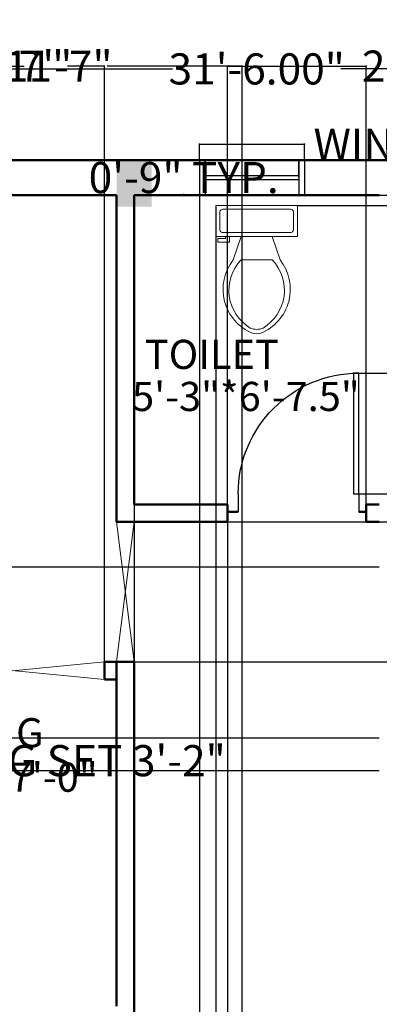
# Model space of a CAD drawing. Units: inches. Extents: x 9717 to 10218, y 17835 to 18358.
# Tile 3 of 4: x 9901 to 9993, y 18104 to 18358. Entities that reach past the tile are written whole.
import ezdxf

# ---------------------------------------------------------------- set-up
doc = ezdxf.new("R2010")
doc.units = ezdxf.units.IN
for name, color, linetype, lineweight in [('A-AREA-IDEN', 3, 'Continuous', 25), ('A-FLOR-FIXT', 2, 'Continuous', 18), ('ARCHES', 5, 'Continuous', 18), ('COLUMN', 7, 'Continuous', 35), ('DIMENSIONS', 3, 'Continuous', 18), ('DOORS', 1, 'Continuous', 25), ('WALLS', 7, 'Continuous', 50), ('WINDOWS', 4, 'Continuous', 25)]:
    doc.layers.add(name, color=color, linetype=linetype, lineweight=lineweight)
doc.styles.get("Standard").update_dxf_attribs({"font": 'arial.ttf'})
doc.dimstyles.get("Standard").update_dxf_attribs({"dimtxt": 8, "dimasz": 0.18, "dimexe": 0.18, "dimexo": 0.0625, "dimgap": 0.09, "dimtad": 0, "dimtih": 1, "dimtoh": 1, "dimzin": 0, "dimdsep": 46, "dimlunit": 3, "dimtxsty": 'Standard', "dimcen": 0.09, "dimadec": 0, "dimazin": 0, "dimtfac": 1, "dimtofl": 0, "dimtmove": 0, "dimatfit": 3, "dimfxl": 1, "dimtolj": 1, "dimtzin": 0, "dimarcsym": 0})

# ---------------------------------------------------------------- blocks, each defined once
blk = doc.blocks.new('*U2')
for p, q in [((0, 0), (0, -6)), ((40, 0), (40, -6))]:
    blk.add_line(p, q)
blk.add_lwpolyline([(0, 0), (0, 40), (1.75, 40), (1.75, 0)], close=True)
blk.add_arc((0, 0), 40, 0, 90)
blk = doc.blocks.new('Toilet - top')
for p, q in [((9.5, -6), (9.5, -2)), ((-10, -8.5), (-8, -8.5)), ((-10, -9.5), (-10, -8.5)), ((-7, -9.5), (-10, -9.5)), ((-8, -8.5), (-8, -8)), ((-7, -8), (-7, -9.5)), ((-4, -8), (-6, -14)), ((4, -8), (6, -14)), ((4, -14), (-4, -14))]:
    blk.add_line(p, q)
blk.add_lwpolyline([(10.5, -8), (10.5, 0), (-10.5, 0), (-10.5, -8)], close=True)
for points in [[(-9.5, -2), (-9.5, -6)], [(8.5, -1), (-8.5, -1)], [(-8.5, -7), (8.5, -7)]]:
    blk.add_lwpolyline(points)
for centre, radius, start, end in [((-8.62, -1.88), 0.884, 81.8699, 188.1301), ((8.62, -1.88), 0.884, 351.8699, 98.1301), ((-8.62, -6.12), 0.884, 171.8699, 278.1301), ((8.62, -6.12), 0.884, 261.8699, 8.1301), ((3.52, -21.58), 12.17, 141.4691, 247.9714), ((4.2, -21.82), 11.33, 136.3677, 238.9468), ((-3.52, -21.58), 12.17, 292.0284, 38.5307), ((-4.2, -21.82), 11.33, 301.053, 43.6321), ((0, -27.88), 4, 245.7318, 294.2682), ((0, -29), 4, 254.8605, 285.1395)]:
    blk.add_arc(centre, radius, start, end)
blk = doc.blocks.new('*D8')
at = {"layer": 'Defpoints', "color": 0, "transparency": 16777216}
for p in [(10150.76, 18344.92), (9772.76, 18321.49), (10150.76, 18321.49)]:
    blk.add_point(p, dxfattribs=at)
at = {"layer": 'DIMENSIONS', "color": 0, "lineweight": -2, "transparency": 16777216}
for p, q in [((9772.76, 18321.55), (9772.76, 18345.1)), ((9772.94, 18344.92), (9940.16, 18344.92)), ((10150.58, 18344.92), (9983.36, 18344.92)), ((10150.76, 18321.55), (10150.76, 18345.1))]:
    blk.add_line(p, q, dxfattribs=at)
at = {"layer": 'DIMENSIONS', "color": 0, "transparency": 16777216}
for points in [[(9772.94, 18344.95), (9772.94, 18344.89), (9772.76, 18344.92)], [(10150.58, 18344.95), (10150.58, 18344.89), (10150.76, 18344.92)]]:
    blk.add_solid(points, dxfattribs=at)
at = {"layer": 'DIMENSIONS', "color": 0, "transparency": 16777216, "insert": (9961.76, 18344.92), "char_height": 8, "attachment_point": 5}
blk.add_mtext('\\A1;31\'-6.00"', dxfattribs=at)
blk = doc.blocks.new('WIN-24IN')
for p, q in [((1.5, 9), (0, 9)), ((0, 9), (0, 0)), ((1.5, 4.5), (1.5, 9)), ((1.5, 9), (1.5, 0)), ((25.5, 4.5), (25.5, 9)), ((25.5, 9), (25.5, 0)), ((25.5, 9), (27, 9)), ((27, 9), (27, 0)), ((1.5, 5), (25.5, 5)), ((1.5, 4), (25.5, 4)), ((0, 0), (1.5, 0)), ((27, 0), (25.5, 0))]:
    blk.add_line(p, q)
blk = doc.blocks.new('COL-12X9IN')
h = blk.add_hatch(color=256)
h.dxf.hatch_style = 1
h.paths.add_polyline_path([(12, 0), (12, 9), (0, 9), (0, 0)])
blk = doc.blocks.new('*D18')
at = {"layer": 'Defpoints', "color": 0, "transparency": 16777216}
for p in [(9974.05, 18325.54), (9947.05, 18321.49), (9974.05, 18321.49)]:
    blk.add_point(p, dxfattribs=at)
at = {"layer": 'DIMENSIONS', "color": 0, "lineweight": -2, "transparency": 16777216}
for p, q in [((9947.05, 18321.55), (9947.05, 18325.72)), ((9947.23, 18325.54), (9973.87, 18325.54)), ((9974.05, 18321.55), (9974.05, 18325.72)), ((9974.05, 18325.54), (9974.23, 18325.54))]:
    blk.add_line(p, q, dxfattribs=at)
at = {"layer": 'DIMENSIONS', "color": 0, "transparency": 16777216}
for points in [[(9947.23, 18325.57), (9947.23, 18325.51), (9947.05, 18325.54)], [(9973.87, 18325.57), (9973.87, 18325.51), (9974.05, 18325.54)]]:
    blk.add_solid(points, dxfattribs=at)
at = {"layer": 'DIMENSIONS', "color": 0, "transparency": 16777216, "insert": (10024.94, 18325.54), "char_height": 8, "attachment_point": 5}
blk.add_mtext('\\A1;WINDOW 2\'-3" TYP.', dxfattribs=at)
blk = doc.blocks.new('*D19')
at = {"layer": 'Defpoints', "color": 0, "transparency": 16777216}
for p in [(9943, 18321.49), (9947.05, 18321.49), (9947.05, 18312.49)]:
    blk.add_point(p, dxfattribs=at)
at = {"layer": 'DIMENSIONS', "color": 0, "lineweight": -2, "transparency": 16777216}
for p, q in [((9946.99, 18321.49), (9942.82, 18321.49)), ((9943, 18321.31), (9943, 18321.17)), ((9946.99, 18312.49), (9942.82, 18312.49)), ((9943, 18312.67), (9943, 18312.82))]:
    blk.add_line(p, q, dxfattribs=at)
at = {"layer": 'DIMENSIONS', "color": 0, "transparency": 16777216}
for points in [[(9942.97, 18321.31), (9943.03, 18321.31), (9943, 18321.49)], [(9942.97, 18312.67), (9943.03, 18312.67), (9943, 18312.49)]]:
    blk.add_solid(points, dxfattribs=at)
at = {"layer": 'DIMENSIONS', "color": 0, "transparency": 16777216, "insert": (9943, 18316.99), "char_height": 8, "attachment_point": 5}
blk.add_mtext('\\A1;0\'-9" TYP.', dxfattribs=at)
blk = doc.blocks.new('*D28')
at = {"layer": 'Defpoints', "color": 0, "transparency": 16777216}
for p in [(9866.73, 18167.12), (9828.75, 18161.43), (9866.73, 18161.43)]:
    blk.add_point(p, dxfattribs=at)
at = {"layer": 'DIMENSIONS', "color": 0, "lineweight": -2, "transparency": 16777216}
for p, q in [((9828.75, 18161.49), (9828.75, 18167.3)), ((9828.93, 18167.12), (9866.55, 18167.12)), ((9866.73, 18161.49), (9866.73, 18167.3)), ((9866.73, 18167.12), (9866.91, 18167.12))]:
    blk.add_line(p, q, dxfattribs=at)
at = {"layer": 'DIMENSIONS', "color": 0, "transparency": 16777216}
for points in [[(9828.93, 18167.15), (9828.93, 18167.09), (9828.75, 18167.12)], [(9866.55, 18167.15), (9866.55, 18167.09), (9866.73, 18167.12)]]:
    blk.add_solid(points, dxfattribs=at)
at = {"layer": 'DIMENSIONS', "color": 0, "transparency": 16777216, "insert": (9910.97, 18167.12), "char_height": 8, "attachment_point": 5}
blk.add_mtext('\\A1;DINING SET 3\'-2"', dxfattribs=at)
blk = doc.blocks.new('*D33')
at = {"layer": 'Defpoints', "color": 0, "transparency": 16777216}
for p in [(9958.06, 18345.64), (9867.28, 17970.49), (9958.06, 17970.49)]:
    blk.add_point(p, dxfattribs=at)
at = {"layer": 'DIMENSIONS', "color": 0, "lineweight": -2, "transparency": 16777216}
for p, q in [((9867.28, 17970.55), (9867.28, 18345.82)), ((9958.06, 17970.55), (9958.06, 18345.82)), ((9867.46, 18345.64), (9901.98, 18345.64)), ((9957.88, 18345.64), (9923.36, 18345.64))]:
    blk.add_line(p, q, dxfattribs=at)
at = {"layer": 'DIMENSIONS', "color": 0, "transparency": 16777216}
for points in [[(9867.46, 18345.67), (9867.46, 18345.61), (9867.28, 18345.64)], [(9957.88, 18345.67), (9957.88, 18345.61), (9958.06, 18345.64)]]:
    blk.add_solid(points, dxfattribs=at)
at = {"layer": 'DIMENSIONS', "color": 0, "transparency": 16777216, "insert": (9912.67, 18345.64), "char_height": 8, "attachment_point": 5}
blk.add_mtext('\\A1;7\'-7"', dxfattribs=at)
blk = doc.blocks.new('*D41')
at = {"layer": 'Defpoints', "color": 0, "transparency": 16777216}
for p in [(9930.26, 18312.49), (9947.05, 18312.49), (9947.05, 17847.34)]:
    blk.add_point(p, dxfattribs=at)
at = {"layer": 'DIMENSIONS', "color": 0, "lineweight": -2, "transparency": 16777216}
for p, q in [((9930.26, 18312.43), (9930.26, 17847.16)), ((9947.05, 18312.43), (9947.05, 17847.16)), ((9930.44, 17847.34), (9946.87, 17847.34)), ((9947.05, 17847.34), (9947.23, 17847.34))]:
    blk.add_line(p, q, dxfattribs=at)
at = {"layer": 'DIMENSIONS', "color": 0, "transparency": 16777216}
for points in [[(9930.44, 17847.37), (9930.44, 17847.31), (9930.26, 17847.34)], [(9946.87, 17847.37), (9946.87, 17847.31), (9947.05, 17847.34)]]:
    blk.add_solid(points, dxfattribs=at)
at = {"layer": 'DIMENSIONS', "color": 0, "transparency": 16777216, "insert": (9957.58, 17847.34), "char_height": 8, "attachment_point": 5}
blk.add_mtext('\\A1;1\'-5"', dxfattribs=at)
blk = doc.blocks.new('*D49')
at = {"layer": 'Defpoints', "color": 0, "transparency": 16777216}
for p in [(9922.68, 18345.64), (9875.9, 18192.49), (9922.68, 18192.49)]:
    blk.add_point(p, dxfattribs=at)
at = {"layer": 'DIMENSIONS', "color": 0, "lineweight": -2, "transparency": 16777216}
for p, q in [((9875.9, 18192.55), (9875.9, 18345.82)), ((9922.68, 18192.55), (9922.68, 18345.82)), ((9876.08, 18345.64), (9885.46, 18345.64)), ((9922.5, 18345.64), (9913.12, 18345.64))]:
    blk.add_line(p, q, dxfattribs=at)
at = {"layer": 'DIMENSIONS', "color": 0, "transparency": 16777216}
for points in [[(9876.08, 18345.67), (9876.08, 18345.61), (9875.9, 18345.64)], [(9922.5, 18345.67), (9922.5, 18345.61), (9922.68, 18345.64)]]:
    blk.add_solid(points, dxfattribs=at)
at = {"layer": 'DIMENSIONS', "color": 0, "transparency": 16777216, "insert": (9899.29, 18345.64), "char_height": 8, "attachment_point": 5}
blk.add_mtext('\\A1;3\'-11"', dxfattribs=at)
blk = doc.blocks.new('*D50')
at = {"layer": 'Defpoints', "color": 0, "transparency": 16777216}
for p in [(9930.26, 18228.49), (10174.91, 18228.49), (9930.26, 18192.49)]:
    blk.add_point(p, dxfattribs=at)
at = {"layer": 'DIMENSIONS', "color": 0, "lineweight": -2, "transparency": 16777216}
for p, q in [((9930.32, 18228.49), (10175.09, 18228.49)), ((10174.91, 18228.31), (10174.91, 18214.67)), ((10174.91, 18192.67), (10174.91, 18206.31)), ((9930.32, 18192.49), (10175.09, 18192.49))]:
    blk.add_line(p, q, dxfattribs=at)
at = {"layer": 'DIMENSIONS', "color": 0, "transparency": 16777216}
for points in [[(10174.88, 18228.31), (10174.94, 18228.31), (10174.91, 18228.49)], [(10174.88, 18192.67), (10174.94, 18192.67), (10174.91, 18192.49)]]:
    blk.add_solid(points, dxfattribs=at)
at = {"layer": 'DIMENSIONS', "color": 0, "transparency": 16777216, "insert": (10174.91, 18210.49), "char_height": 8, "attachment_point": 5}
blk.add_mtext('\\A1;3\'-0"', dxfattribs=at)
blk = doc.blocks.new('*D51')
at = {"layer": 'Defpoints', "color": 0, "transparency": 16777216}
for p in [(9989.89, 18345.64), (9954.27, 18232.99), (9989.89, 18232.99)]:
    blk.add_point(p, dxfattribs=at)
at = {"layer": 'DIMENSIONS', "color": 0, "lineweight": -2, "transparency": 16777216}
for p, q in [((9954.27, 18233.05), (9954.27, 18345.82)), ((9989.89, 18233.05), (9989.89, 18345.82)), ((9954.45, 18345.64), (9989.71, 18345.64)), ((9989.89, 18345.64), (9990.07, 18345.64))]:
    blk.add_line(p, q, dxfattribs=at)
at = {"layer": 'DIMENSIONS', "color": 0, "transparency": 16777216}
for points in [[(9954.45, 18345.67), (9954.45, 18345.61), (9954.27, 18345.64)], [(9989.71, 18345.67), (9989.71, 18345.61), (9989.89, 18345.64)]]:
    blk.add_solid(points, dxfattribs=at)
at = {"layer": 'DIMENSIONS', "color": 0, "transparency": 16777216, "insert": (10013.29, 18345.64), "char_height": 8, "attachment_point": 5}
blk.add_mtext('\\A1;2\'-11 1/2"', dxfattribs=at)
blk = doc.blocks.new('*D52')
at = {"layer": 'Defpoints', "color": 0, "transparency": 16777216}
for p in [(9748.61, 18216.87), (9993.26, 18216.87), (9993.26, 18172.92)]:
    blk.add_point(p, dxfattribs=at)
at = {"layer": 'DIMENSIONS', "color": 0, "lineweight": -2, "transparency": 16777216}
for p, q in [((9993.2, 18216.87), (9748.43, 18216.87)), ((9748.61, 18216.69), (9748.61, 18199.08)), ((9748.61, 18173.1), (9748.61, 18190.72)), ((9993.2, 18172.92), (9748.43, 18172.92))]:
    blk.add_line(p, q, dxfattribs=at)
at = {"layer": 'DIMENSIONS', "color": 0, "transparency": 16777216}
for points in [[(9748.58, 18216.69), (9748.64, 18216.69), (9748.61, 18216.87)], [(9748.58, 18173.1), (9748.64, 18173.1), (9748.61, 18172.92)]]:
    blk.add_solid(points, dxfattribs=at)
at = {"layer": 'DIMENSIONS', "color": 0, "transparency": 16777216, "insert": (9748.61, 18194.9), "char_height": 8, "attachment_point": 5}
blk.add_mtext('\\A1;3\'-8"', dxfattribs=at)
blk = doc.blocks.new('*D56')
at = {"layer": 'Defpoints', "color": 0, "transparency": 16777216}
for p in [(9986.65, 18266.74), (10174.91, 18266.74), (9986.65, 18235.74)]:
    blk.add_point(p, dxfattribs=at)
at = {"layer": 'DIMENSIONS', "color": 0, "lineweight": -2, "transparency": 16777216}
for p, q in [((9986.71, 18266.74), (10175.09, 18266.74)), ((10174.91, 18266.56), (10174.91, 18255.34)), ((10174.91, 18235.92), (10174.91, 18247.13)), ((9986.71, 18235.74), (10175.09, 18235.74))]:
    blk.add_line(p, q, dxfattribs=at)
at = {"layer": 'DIMENSIONS', "color": 0, "transparency": 16777216}
for points in [[(10174.88, 18266.56), (10174.94, 18266.56), (10174.91, 18266.74)], [(10174.88, 18235.92), (10174.94, 18235.92), (10174.91, 18235.74)]]:
    blk.add_solid(points, dxfattribs=at)
at = {"layer": 'DIMENSIONS', "color": 0, "transparency": 16777216, "insert": (10174.91, 18251.24), "char_height": 8, "attachment_point": 5}
blk.add_mtext('\\A1;2\'-7"', dxfattribs=at)
blk = doc.blocks.new('*D58')
at = {"layer": 'Defpoints', "color": 0, "transparency": 16777216}
for p in [(9930.26, 18232.99), (9954.27, 18232.99), (9954.27, 17847.34)]:
    blk.add_point(p, dxfattribs=at)
at = {"layer": 'DIMENSIONS', "color": 0, "lineweight": -2, "transparency": 16777216}
for p, q in [((9930.26, 18232.93), (9930.26, 17847.16)), ((9954.27, 18232.93), (9954.27, 17847.16)), ((9930.44, 17847.34), (9931.48, 17847.34)), ((9954.09, 17847.34), (9953.06, 17847.34))]:
    blk.add_line(p, q, dxfattribs=at)
at = {"layer": 'DIMENSIONS', "color": 0, "transparency": 16777216}
for points in [[(9930.44, 17847.37), (9930.44, 17847.31), (9930.26, 17847.34)], [(9954.09, 17847.37), (9954.09, 17847.31), (9954.27, 17847.34)]]:
    blk.add_solid(points, dxfattribs=at)
at = {"layer": 'DIMENSIONS', "color": 0, "transparency": 16777216, "insert": (9942.27, 17847.34), "char_height": 8, "attachment_point": 5}
blk.add_mtext('\\A1;2\'-0"', dxfattribs=at)
blk = doc.blocks.new('*D61')
at = {"layer": 'Defpoints', "color": 0, "transparency": 16777216}
for p in [(9748.61, 18172.92), (9993.26, 18172.92), (9993.26, 18164.49)]:
    blk.add_point(p, dxfattribs=at)
at = {"layer": 'DIMENSIONS', "color": 0, "lineweight": -2, "transparency": 16777216}
for p, q in [((9993.2, 18172.92), (9748.43, 18172.92)), ((9748.61, 18172.92), (9748.61, 18173.1)), ((9748.61, 18173.1), (9748.79, 18173.1)), ((9748.61, 18164.67), (9748.61, 18172.74)), ((9993.2, 18164.49), (9748.43, 18164.49))]:
    blk.add_line(p, q, dxfattribs=at)
at = {"layer": 'DIMENSIONS', "color": 0, "transparency": 16777216}
for points in [[(9748.58, 18172.74), (9748.64, 18172.74), (9748.61, 18172.92)], [(9748.58, 18164.67), (9748.64, 18164.67), (9748.61, 18164.49)]]:
    blk.add_solid(points, dxfattribs=at)
at = {"layer": 'DIMENSIONS', "color": 0, "transparency": 16777216, "insert": (9768.83, 18173.1), "char_height": 8, "attachment_point": 5}
blk.add_mtext('\\A1;0\'-8 1/2"', dxfattribs=at)
blk = doc.blocks.new('*D64')
at = {"layer": 'Defpoints', "color": 0, "transparency": 16777216}
for p in [(9930.26, 18312.49), (9951.25, 18309.85), (9951.25, 17847.34)]:
    blk.add_point(p, dxfattribs=at)
at = {"layer": 'DIMENSIONS', "color": 0, "lineweight": -2, "transparency": 16777216}
for p, q in [((9930.26, 18312.43), (9930.26, 17847.16)), ((9951.25, 18309.78), (9951.25, 17847.16)), ((9930.08, 17847.34), (9929.9, 17847.34)), ((9951.43, 17847.34), (9951.61, 17847.34))]:
    blk.add_line(p, q, dxfattribs=at)
at = {"layer": 'DIMENSIONS', "color": 0, "transparency": 16777216}
for points in [[(9930.08, 17847.37), (9930.08, 17847.31), (9930.26, 17847.34)], [(9951.43, 17847.37), (9951.43, 17847.31), (9951.25, 17847.34)]]:
    blk.add_solid(points, dxfattribs=at)
at = {"layer": 'DIMENSIONS', "color": 0, "transparency": 16777216, "insert": (9940.75, 17847.34), "char_height": 8, "attachment_point": 5}
blk.add_mtext('\\A1;1\'-9"', dxfattribs=at)
blk = doc.blocks.new('*D67')
at = {"layer": 'Defpoints', "color": 0, "transparency": 16777216}
for p in [(9974.05, 18312.49), (10174.91, 18312.49), (9972.25, 18309.85)]:
    blk.add_point(p, dxfattribs=at)
at = {"layer": 'DIMENSIONS', "color": 0, "lineweight": -2, "transparency": 16777216}
for p, q in [((9974.12, 18312.49), (10175.09, 18312.49)), ((10174.91, 18312.49), (10174.91, 18312.67)), ((10174.91, 18312.67), (10175.09, 18312.67)), ((10174.91, 18310.03), (10174.91, 18312.31)), ((9972.31, 18309.85), (10175.09, 18309.85))]:
    blk.add_line(p, q, dxfattribs=at)
at = {"layer": 'DIMENSIONS', "color": 0, "transparency": 16777216}
for points in [[(10174.88, 18312.31), (10174.94, 18312.31), (10174.91, 18312.49)], [(10174.88, 18310.03), (10174.94, 18310.03), (10174.91, 18309.85)]]:
    blk.add_solid(points, dxfattribs=at)
at = {"layer": 'DIMENSIONS', "color": 0, "transparency": 16777216, "insert": (10195.13, 18312.67), "char_height": 8, "attachment_point": 5}
blk.add_mtext('\\A1;0\'-2 1/2"', dxfattribs=at)

msp = doc.modelspace()

# ---------------------------------------------------------------- linework, layer by layer
at = {"layer": 'ARCHES'}
for p, q in [((9930.26, 18192.491), (9925.76, 18228.491)), ((9925.76, 18228.491), (9930.26, 18228.491)), ((9930.26, 18228.491), (9925.76, 18192.491)), ((9875.896, 18192.491), (9922.682, 18187.991)), ((9922.682, 18192.491), (9875.896, 18187.991)), ((9925.76, 18192.491), (9930.26, 18192.491))]:
    msp.add_line(p, q, dxfattribs=at)
at = {"layer": 'WALLS'}
for p, q in [((9781.76, 18312.491), (9925.76, 18312.491)), ((9925.76, 18228.491), (9925.76, 18312.491)), ((9930.26, 18312.491), (9993.26, 18312.491)), ((9930.26, 18232.991), (9930.26, 18312.491)), ((9930.26, 18232.991), (9954.275, 18232.991)), ((9954.275, 18232.991), (9954.275, 18228.491)), ((9989.894, 18232.991), (9989.894, 18228.491)), ((9989.894, 18232.991), (9993.26, 18232.991)), ((9957.005, 18231.086), (9954.275, 18231.086)), ((9988.005, 18231.086), (9989.894, 18231.086)), ((9925.76, 18228.491), (9954.275, 18228.491)), ((9989.894, 18228.491), (9993.26, 18228.491)), ((9922.682, 18187.991), (9922.682, 18192.491)), ((9922.682, 18187.991), (9922.682, 18192.491)), ((9925.76, 18192.491), (9922.682, 18192.491)), ((9922.682, 18192.491), (9922.682, 18187.991)), ((9925.76, 18103.991), (9925.76, 18192.491)), ((9925.76, 18192.491), (9930.26, 18192.491)), ((9930.26, 18099.491), (9930.26, 18192.491)), ((9922.682, 18187.991), (9925.76, 18187.991))]:
    msp.add_line(p, q, dxfattribs=at)
msp.add_lwpolyline([(9867.276, 17961.491), (9772.76, 17961.491), (9772.76, 18321.491), (10150.76, 18321.491), (10150.76, 17961.491)], dxfattribs=at)

# ---------------------------------------------------------------- block references
at = {"layer": 'A-FLOR-FIXT'}
msp.add_blockref('Toilet - top', (9961.746, 18309.847), dxfattribs=at)
at = {"layer": 'COLUMN', "rotation": 269.9999999999907}
msp.add_blockref('COL-12X9IN', (9925.734, 18321.492), dxfattribs=at)
at = {"layer": 'DOORS', "xscale": -0.775, "yscale": 0.775, "zscale": 0.775}
msp.add_blockref('*U2', (9988.005, 18235.736), dxfattribs=at)
at = {"layer": 'WINDOWS'}
msp.add_blockref('WIN-24IN', (9947.053, 18312.491), dxfattribs=at)

# ---------------------------------------------------------------- texts
at = {"layer": 'A-AREA-IDEN'}
for s, p in [('TOILET', (9933.017, 18267.793)), ('5\'-3"*6\'-7.5"', (9929.724, 18256.981)), ('DINNING', (9864.707, 18170.542)), ('12\'-0" * 7\'-0"', (9860.657, 18159.128))]:
    msp.add_text(s, height=7.5, dxfattribs=at).set_placement(p)

# ---------------------------------------------------------------- dimensions: what is measured, and where the dimension line sits
at = {"layer": 'DIMENSIONS'}
for base, p1, p2, override, picture, middle in [((9989.894, 18345.641), (9954.275, 18232.991), (9989.894, 18232.991), {"dimdec": 1, "dimlfac": 1, "dimrnd": 0, "dimzin": 1, "dimdsep": 46, "dimlunit": 4, "dimfrac": 2}, '*D51', (10013.293, 18345.641)), ((9958.06, 18345.641), (9867.276, 17970.491), (9958.06, 17970.491), {"dimdec": 1, "dimlfac": 1, "dimrnd": 0, "dimzin": 1, "dimdsep": 46, "dimlunit": 4, "dimfrac": 2}, '*D33', (9912.668, 18345.641)), ((9922.682, 18345.641), (9875.896, 18192.491), (9922.682, 18192.491), {"dimdec": 1, "dimlfac": 1, "dimrnd": 0, "dimzin": 1, "dimdsep": 46, "dimlunit": 4, "dimfrac": 2}, '*D49', (9899.289, 18345.641)), ((10150.76, 18344.922), (9772.76, 18321.491), (10150.76, 18321.491), {"dimclrd": 0, "dimclre": 0, "dimclrt": 0}, '*D8', (9961.76, 18344.922)), ((9951.246, 17847.341), (9930.26, 18312.491), (9951.246, 18309.847), {"dimdec": 1, "dimlfac": 1, "dimrnd": 0, "dimzin": 1, "dimdsep": 46, "dimlunit": 4, "dimfrac": 2}, '*D64', (9940.753, 17847.341)), ((9947.053, 17847.341), (9930.26, 18312.491), (9947.053, 18312.491), {"dimdec": 1, "dimlfac": 1, "dimrnd": 0, "dimzin": 1, "dimdsep": 46, "dimlunit": 4, "dimfrac": 2}, '*D41', (9957.579, 17847.341)), ((9954.275, 17847.341), (9930.26, 18232.991), (9954.275, 18232.991), {"dimdec": 1, "dimlfac": 1, "dimrnd": 0, "dimzin": 1, "dimdsep": 46, "dimlunit": 4, "dimfrac": 2}, '*D58', (9942.268, 17847.341))]:
    dim = msp.add_linear_dim(base=base, p1=p1, p2=p2, dimstyle='Standard', override=override, dxfattribs=at)
    dim.commit()
    dim.dimension.update_dxf_attribs({"geometry": picture, "text_midpoint": middle})
for base, p1, p2, text, picture, middle in [((9974.053, 18325.541), (9947.053, 18321.491), (9974.053, 18321.491), 'WINDOW <> TYP.', '*D18', (10024.939, 18325.541)), ((9866.734, 18167.124), (9828.75, 18161.426), (9866.734, 18161.426), 'DINING SET <>', '*D28', (9910.968, 18167.124))]:
    dim = msp.add_linear_dim(base=base, p1=p1, p2=p2, text=text, dimstyle='Standard', override={"dimdec": 1, "dimlfac": 1, "dimrnd": 0, "dimzin": 1, "dimdsep": 46, "dimlunit": 4, "dimfrac": 2}, dxfattribs=at)
    dim.commit()
    dim.dimension.update_dxf_attribs({"geometry": picture, "text_midpoint": middle})
dim = msp.add_linear_dim(base=(9943.003, 18321.491), p1=(9947.053, 18312.491), p2=(9947.053, 18321.491), angle=90, text='<> TYP.', dimstyle='Standard', override={"dimdec": 1, "dimlfac": 1, "dimrnd": 0, "dimzin": 1, "dimdsep": 46, "dimlunit": 4, "dimfrac": 2}, dxfattribs=at)
dim.commit()
dim.dimension.update_dxf_attribs({"geometry": '*D19', "text_midpoint": (9943.003, 18316.991)})
for base, p1, p2, picture, middle in [((10174.91, 18312.491), (9972.246, 18309.847), (9974.053, 18312.491), '*D67', (10195.134, 18312.671)), ((10174.91, 18266.736), (9986.649, 18235.736), (9986.649, 18266.736), '*D56', (10174.91, 18251.236)), ((10174.91, 18228.491), (9930.26, 18192.491), (9930.26, 18228.491), '*D50', (10174.91, 18210.491)), ((9748.61, 18216.874), (9993.26, 18172.923), (9993.26, 18216.874), '*D52', (9748.61, 18194.899)), ((9748.61, 18172.923), (9993.26, 18164.491), (9993.26, 18172.923), '*D61', (9768.834, 18173.103))]:
    dim = msp.add_linear_dim(base=base, p1=p1, p2=p2, angle=90, dimstyle='Standard', override={"dimdec": 1, "dimlfac": 1, "dimrnd": 0, "dimzin": 1, "dimdsep": 46, "dimlunit": 4, "dimfrac": 2}, dxfattribs=at)
    dim.commit()
    dim.dimension.update_dxf_attribs({"geometry": picture, "text_midpoint": middle})

doc.saveas('drawing.dxf')
